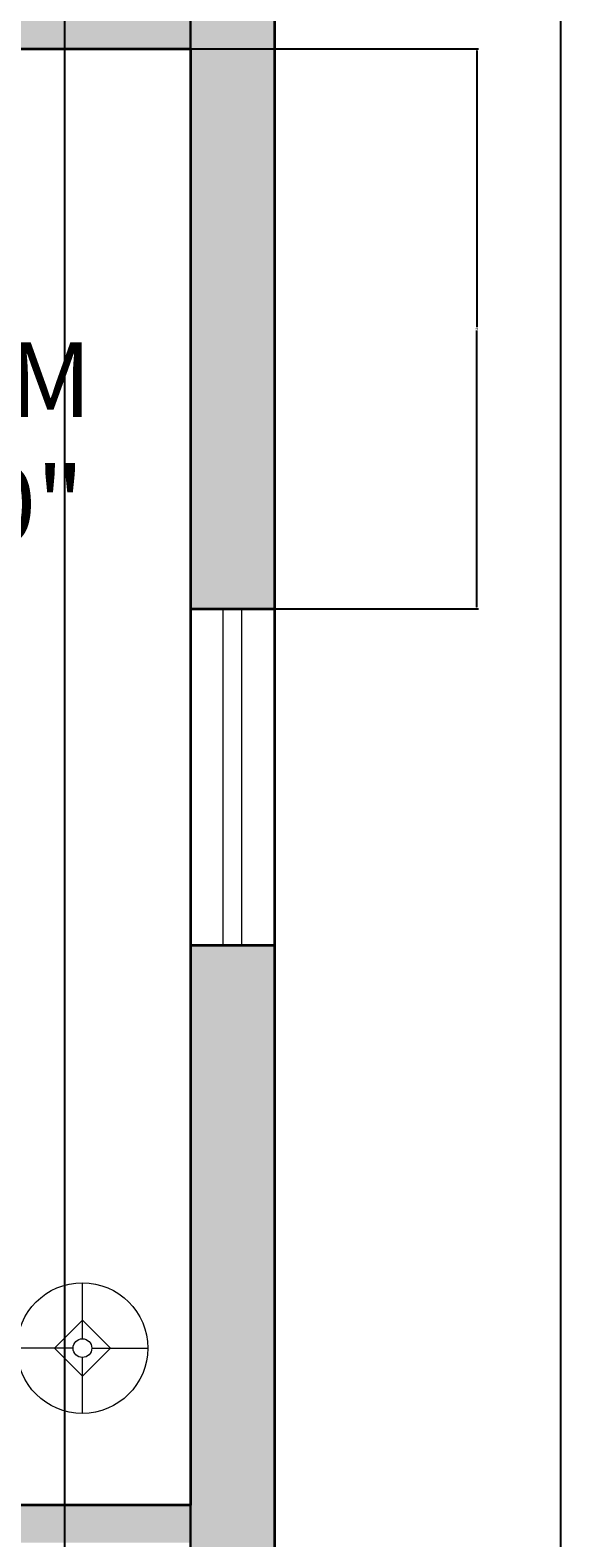
# Model space of a CAD drawing. Units: inches. Extents: x 1567 to 1964, y 1813 to 2447.
# Tile 6 of 28: x 1907 to 1964, y 1964 to 2125. Entities that reach past the tile are written whole.
import ezdxf

# ---------------------------------------------------------------- set-up
doc = ezdxf.new("R2010")
doc.units = ezdxf.units.IN
for name, color, linetype, lineweight in [('A-ANNO-DIMS', 2, 'Continuous', 18), ('A-AREA-IDEN', 7, 'Continuous', 18), ('A-FURN', 8, 'Continuous', 18), ('A-GLAZ', 4, 'Continuous', 18), ('A-WALL', 7, 'Continuous', 35)]:
    doc.layers.add(name, color=color, linetype=linetype, lineweight=lineweight)
doc.layers.add('A-FURN-PATT', color=252, linetype='Continuous', lineweight=13, true_color=0x939598)
doc.layers.add('A-WALL-PATT', color=251, linetype='Continuous', lineweight=13, true_color=0x636466)
doc.styles.get("Standard").update_dxf_attribs({"font": 'arial.ttf'})
doc.dimstyles.get("Standard").update_dxf_attribs({"dimtxt": 0.18, "dimasz": 0.18, "dimexe": 0.18, "dimexo": 0.0625, "dimgap": 0.09, "dimtad": 0, "dimtih": 1, "dimtoh": 1, "dimdec": 4, "dimzin": 0, "dimdsep": 46, "dimtxsty": 'Standard', "dimcen": 0.09, "dimadec": 0, "dimazin": 0, "dimtfac": 1, "dimtdec": 4, "dimtofl": 0, "dimtmove": 0, "dimatfit": 3, "dimfxl": 1, "dimtolj": 1, "dimtzin": 0, "dimarcsym": 0})

# ---------------------------------------------------------------- blocks, each defined once
blk = doc.blocks.new('Lamp - Table')
for p, q in [((0, 7), (0, 1)), ((0, 3), (-3, 0)), ((3, 0), (0, 3)), ((-1, 0), (-7, 0)), ((-3, 0), (0, -3)), ((0, -3), (3, 0)), ((1, 0), (7, 0)), ((0, -1), (0, -7))]:
    blk.add_line(p, q)
for radius in [7, 1]:
    blk.add_circle((0, 0), radius)
blk = doc.blocks.new('WINDOW-36IN')
for p, q in [((0, 2), (36, 2)), ((0, 0), (36, 0))]:
    blk.add_line(p, q)
blk = doc.blocks.new('*D40')
at = {"layer": 'A-ANNO-DIMS', "color": 0, "lineweight": -2, "transparency": 16777216}
for p, q in [((1933.49, 2416.29), (1964.26, 2416.29)), ((1964.08, 2416.11), (1964.08, 2130.47)), ((1964.08, 1844.47), (1964.08, 2130.11)), ((1933.49, 1844.29), (1964.26, 1844.29))]:
    blk.add_line(p, q, dxfattribs=at)
at = {"layer": 'A-ANNO-DIMS', "color": 0, "transparency": 16777216}
for points in [[(1964.05, 2416.11), (1964.11, 2416.11), (1964.08, 2416.29)], [(1964.05, 1844.47), (1964.11, 1844.47), (1964.08, 1844.29)]]:
    blk.add_solid(points, dxfattribs=at)
at = {"layer": 'Defpoints', "color": 0, "transparency": 16777216}
for p in [(1933.43, 2416.29), (1964.08, 2416.29), (1933.43, 1844.29)]:
    blk.add_point(p, dxfattribs=at)
at = {"layer": 'A-ANNO-DIMS', "color": 0, "transparency": 16777216, "insert": (1964.08, 2130.29), "char_height": 0.18, "attachment_point": 5}
blk.add_mtext('\\A1;572', dxfattribs=at)
blk = doc.blocks.new('*D52')
at = {"layer": 'A-ANNO-DIMS', "color": 0, "lineweight": -2, "transparency": 16777216}
for p, q in [((1924.49, 2123.29), (1955.26, 2123.29)), ((1955.08, 2123.11), (1955.08, 2093.47)), ((1955.08, 2063.47), (1955.08, 2093.11)), ((1924.49, 2063.29), (1955.26, 2063.29))]:
    blk.add_line(p, q, dxfattribs=at)
at = {"layer": 'A-ANNO-DIMS', "color": 0, "transparency": 16777216}
for points in [[(1955.05, 2123.11), (1955.11, 2123.11), (1955.08, 2123.29)], [(1955.05, 2063.47), (1955.11, 2063.47), (1955.08, 2063.29)]]:
    blk.add_solid(points, dxfattribs=at)
at = {"layer": 'Defpoints', "color": 0, "transparency": 16777216}
for p in [(1924.43, 2123.29), (1924.43, 2063.29), (1955.08, 2063.29)]:
    blk.add_point(p, dxfattribs=at)
at = {"layer": 'A-ANNO-DIMS', "color": 0, "transparency": 16777216, "insert": (1955.08, 2093.29), "char_height": 0.18, "attachment_point": 5}
blk.add_mtext('\\A1;60', dxfattribs=at)
blk = doc.blocks.new('*D71')
at = {"layer": 'A-ANNO-DIMS', "color": 0, "lineweight": -2, "transparency": 16777216}
for p, q in [((1799.43, 1910.75), (1799.43, 2447.12)), ((1799.61, 2446.94), (1861.65, 2446.94)), ((1924.25, 2446.94), (1862.21, 2446.94)), ((1924.43, 1910.75), (1924.43, 2447.12))]:
    blk.add_line(p, q, dxfattribs=at)
at = {"layer": 'A-ANNO-DIMS', "color": 0, "transparency": 16777216}
for points in [[(1799.61, 2446.97), (1799.61, 2446.91), (1799.43, 2446.94)], [(1924.25, 2446.97), (1924.25, 2446.91), (1924.43, 2446.94)]]:
    blk.add_solid(points, dxfattribs=at)
at = {"layer": 'Defpoints', "color": 0, "transparency": 16777216}
for p in [(1924.43, 2446.94), (1799.43, 1910.69), (1924.43, 1910.69)]:
    blk.add_point(p, dxfattribs=at)
at = {"layer": 'A-ANNO-DIMS', "color": 0, "transparency": 16777216, "insert": (1861.93, 2446.94), "char_height": 0.18, "attachment_point": 5}
blk.add_mtext('\\A1;125', dxfattribs=at)
blk = doc.blocks.new('*D72')
at = {"layer": 'A-ANNO-DIMS', "color": 0, "lineweight": -2, "transparency": 16777216}
for p, q in [((1910.93, 2175.23), (1910.93, 1813.46)), ((1924.43, 2175.23), (1924.43, 1813.46)), ((1911.11, 1813.64), (1917.36, 1813.64)), ((1924.25, 1813.64), (1918, 1813.64))]:
    blk.add_line(p, q, dxfattribs=at)
at = {"layer": 'A-ANNO-DIMS', "color": 0, "transparency": 16777216}
for points in [[(1911.11, 1813.67), (1911.11, 1813.61), (1910.93, 1813.64)], [(1924.25, 1813.67), (1924.25, 1813.61), (1924.43, 1813.64)]]:
    blk.add_solid(points, dxfattribs=at)
at = {"layer": 'Defpoints', "color": 0, "transparency": 16777216}
for p in [(1910.93, 2175.29), (1924.43, 2175.29), (1924.43, 1813.64)]:
    blk.add_point(p, dxfattribs=at)
at = {"layer": 'A-ANNO-DIMS', "color": 0, "transparency": 16777216, "insert": (1917.68, 1813.64), "char_height": 0.18, "attachment_point": 5}
blk.add_mtext('\\A1;13.5', dxfattribs=at)

msp = doc.modelspace()

# ---------------------------------------------------------------- hatches: boundary and pattern name
at = {"layer": 'A-FURN-PATT'}
h = msp.add_hatch(color=256, dxfattribs=at)
h.dxf.hatch_style = 1
h.paths.add_polyline_path([(1697.3402, 2374.8316), (1682.1402, 2374.8316), (1682.1402, 2387.6316), (1637.3402, 2387.6316), (1637.3402, 2324.4315), (1697.3402, 2324.4315)])
h.paths.add_polyline_path([(1891.1093, 2375.8204), (1875.9094, 2375.8204), (1875.9094, 2388.6204), (1831.1094, 2388.6204), (1831.1094, 2325.4204), (1891.1093, 2325.4204)])
h.paths.add_polyline_path([(1702.5611, 2206.8057), (1702.5611, 2210.8057), (1699.7395, 2209.9436), (1697.013, 2209.2403), (1694.3857, 2208.6763), (1691.8615, 2208.2326), (1689.4443, 2207.8896), (1687.1381, 2207.6282), (1684.9469, 2207.4289), (1682.8747, 2207.2725), (1680.9233, 2207.1425), (1679.0865, 2207.0339), (1677.3558, 2206.9445), (1675.7229, 2206.8719), (1674.1794, 2206.8141), (1672.7169, 2206.7688), (1671.327, 2206.7339), (1670.0014, 2206.707), (1668.7314, 2206.6866), (1667.5072, 2206.6732), (1666.3188, 2206.668), (1665.1561, 2206.6722), (1664.009, 2206.6869), (1662.8675, 2206.7133), (1661.7215, 2206.7525), (1660.5611, 2206.8057), (1660.5611, 2202.8057), (1661.9932, 2202.9556), (1663.3314, 2203.0744), (1664.5899, 2203.1671), (1665.7831, 2203.2385), (1666.9254, 2203.2935), (1668.0311, 2203.3368), (1669.1145, 2203.3734), (1670.1902, 2203.4081), (1671.2724, 2203.4451), (1672.3759, 2203.4866), (1673.5155, 2203.534), (1674.706, 2203.5887), (1675.9621, 2203.6523), (1677.2986, 2203.7262), (1678.7304, 2203.8118), (1680.2722, 2203.9108), (1681.947, 2204.0272), (1683.8108, 2204.1769), (1685.9279, 2204.3782), (1688.3626, 2204.6496), (1691.179, 2205.0096), (1694.4413, 2205.4767), (1698.214, 2206.0692)])
h.paths.add_polyline_path([(1702.5611, 2218.8057), (1701.9821, 2217.9383), (1701.3316, 2217.191), (1700.6091, 2216.5515), (1699.8141, 2216.0071), (1698.946, 2215.5454), (1698.0041, 2215.1536), (1696.9879, 2214.8194), (1695.8969, 2214.5301), (1694.7328, 2214.2753), (1693.5072, 2214.0522), (1692.2339, 2213.8602), (1690.9266, 2213.6989), (1689.5994, 2213.5675), (1688.266, 2213.4654), (1686.9402, 2213.392), (1685.636, 2213.3467), (1684.3619, 2213.3287), (1683.1053, 2213.3361), (1681.8482, 2213.3668), (1680.5727, 2213.4187), (1679.2608, 2213.4898), (1677.8948, 2213.5779), (1676.4565, 2213.6811), (1674.9282, 2213.7971), (1673.2982, 2213.9236), (1671.5804, 2214.0573), (1669.795, 2214.1945), (1667.9622, 2214.3316), (1666.1022, 2214.4649), (1664.2352, 2214.5908), (1662.3814, 2214.7056), (1660.5611, 2214.8057), (1660.5611, 2206.8057), (1661.7215, 2206.7525), (1662.8675, 2206.7133), (1664.009, 2206.6869), (1665.1561, 2206.6722), (1666.3188, 2206.668), (1667.5072, 2206.6732), (1668.7314, 2206.6866), (1670.0014, 2206.707), (1671.327, 2206.7339), (1672.7169, 2206.7688), (1674.1794, 2206.8141), (1675.7229, 2206.8719), (1677.3558, 2206.9445), (1679.0865, 2207.0339), (1680.9233, 2207.1425), (1682.8747, 2207.2725), (1684.9469, 2207.4289), (1687.1381, 2207.6282), (1689.4443, 2207.8896), (1691.8615, 2208.2326), (1694.3857, 2208.6763), (1697.013, 2209.2403), (1699.7395, 2209.9436), (1702.5611, 2210.8057)])
h.paths.add_polyline_path([(1700.6091, 2216.5515), (1701.3316, 2217.191), (1701.9821, 2217.9383), (1702.5611, 2218.8057), (1702.5611, 2222.8057), (1689.452, 2222.8057), (1689.0171, 2222.4556), (1688.4521, 2222.0354), (1687.7806, 2221.5662), (1687.0235, 2221.067), (1686.2019, 2220.5566), (1685.3367, 2220.0541), (1684.4491, 2219.5785), (1683.56, 2219.1486), (1682.6867, 2218.7795), (1681.8312, 2218.4692), (1680.9918, 2218.212), (1680.1667, 2218.0019), (1679.3541, 2217.833), (1678.5524, 2217.6995), (1677.7597, 2217.5954), (1676.9744, 2217.5149), (1676.1942, 2217.4531), (1675.4146, 2217.4093), (1674.6309, 2217.384), (1673.8381, 2217.3774), (1673.0313, 2217.39), (1672.2056, 2217.4221), (1671.3562, 2217.4741), (1670.4782, 2217.5463), (1669.5642, 2217.639), (1668.5968, 2217.7516), (1667.5562, 2217.8833), (1666.4226, 2218.0336), (1665.1761, 2218.2017), (1663.7969, 2218.3869), (1662.2651, 2218.5885), (1660.5611, 2218.8057), (1660.5611, 2214.8057), (1662.3814, 2214.7056), (1664.2352, 2214.5908), (1666.1022, 2214.4649), (1667.9622, 2214.3316), (1669.795, 2214.1945), (1671.5804, 2214.0573), (1673.2982, 2213.9236), (1674.9282, 2213.7971), (1676.4565, 2213.6811), (1677.8948, 2213.5779), (1679.2608, 2213.4898), (1680.5727, 2213.4187), (1681.8482, 2213.3668), (1683.1053, 2213.3361), (1684.3619, 2213.3287), (1685.636, 2213.3467), (1686.9402, 2213.392), (1688.266, 2213.4654), (1689.5994, 2213.5675), (1690.9266, 2213.6989), (1692.2339, 2213.8602), (1693.5072, 2214.0522), (1694.7328, 2214.2753), (1695.8969, 2214.5301), (1696.9879, 2214.8194), (1698.0041, 2215.1536), (1698.946, 2215.5454), (1699.8141, 2216.0071)])
h.paths.add_polyline_path([(1687.0235, 2221.067), (1687.7806, 2221.5662), (1688.4521, 2222.0354), (1689.0171, 2222.4556), (1689.452, 2222.8057), (1660.5611, 2222.8057), (1660.5611, 2218.8057), (1662.2651, 2218.5885), (1663.7969, 2218.3869), (1665.1761, 2218.2017), (1666.4226, 2218.0336), (1667.5562, 2217.8833), (1668.5968, 2217.7516), (1669.5642, 2217.639), (1670.4782, 2217.5463), (1671.3562, 2217.4741), (1672.2056, 2217.4221), (1673.0313, 2217.39), (1673.8381, 2217.3774), (1674.6309, 2217.384), (1675.4146, 2217.4093), (1676.1942, 2217.4531), (1676.9744, 2217.5149), (1677.7597, 2217.5954), (1678.5524, 2217.6995), (1679.3541, 2217.833), (1680.1667, 2218.0019), (1680.9918, 2218.212), (1681.8312, 2218.4692), (1682.6867, 2218.7795), (1683.56, 2219.1486), (1684.4491, 2219.5785), (1685.3367, 2220.0541), (1686.2019, 2220.5566)], flags=17)
h.paths.add_polyline_path([(1702.5611, 2198.8057), (1698.9289, 2199.2412), (1695.8472, 2199.5774), (1693.2166, 2199.8257), (1690.9377, 2199.9973), (1688.9111, 2200.1033), (1687.0375, 2200.155), (1685.2174, 2200.1637), (1683.3514, 2200.1406), (1681.3514, 2200.0941), (1679.1736, 2200.0225), (1676.7858, 2199.921), (1674.1554, 2199.7852), (1671.2502, 2199.6103), (1668.0377, 2199.3919), (1664.4854, 2199.1252), (1660.5611, 2198.8057), (1660.5611, 2194.8057), (1662.2697, 2194.9771), (1663.9673, 2195.0999), (1665.6339, 2195.1809), (1667.2495, 2195.227), (1668.7941, 2195.2449), (1670.2478, 2195.2414), (1671.5906, 2195.2233), (1672.8026, 2195.1974), (1673.8739, 2195.1689), (1674.8359, 2195.1364), (1675.7302, 2195.0967), (1676.5982, 2195.0469), (1677.4817, 2194.9838), (1678.422, 2194.9043), (1679.4609, 2194.8055), (1680.6397, 2194.6842), (1682.005, 2194.5341), (1683.6223, 2194.335), (1685.562, 2194.0637), (1687.8945, 2193.6967), (1690.6902, 2193.2108), (1694.0196, 2192.5826), (1697.9531, 2191.7887), (1702.5611, 2190.8057)])
h.paths.add_polyline_path([(1702.5611, 2206.8057), (1698.214, 2206.0692), (1694.4413, 2205.4767), (1691.179, 2205.0096), (1688.3626, 2204.6496), (1685.9279, 2204.3782), (1683.8108, 2204.1769), (1681.947, 2204.0272), (1680.2722, 2203.9108), (1678.7304, 2203.8118), (1677.2986, 2203.7262), (1675.9621, 2203.6523), (1674.706, 2203.5887), (1673.5155, 2203.534), (1672.3759, 2203.4866), (1671.2724, 2203.4451), (1670.1902, 2203.4081), (1669.1145, 2203.3734), (1668.0311, 2203.3368), (1666.9254, 2203.2935), (1665.7831, 2203.2385), (1664.5899, 2203.1671), (1663.3314, 2203.0744), (1661.9932, 2202.9556), (1660.5611, 2202.8057), (1660.5611, 2198.8057), (1664.4854, 2199.1252), (1668.0377, 2199.3919), (1671.2502, 2199.6103), (1674.1554, 2199.7852), (1676.7858, 2199.921), (1679.1736, 2200.0225), (1681.3514, 2200.0941), (1683.3514, 2200.1406), (1685.2174, 2200.1637), (1687.0375, 2200.155), (1688.9111, 2200.1033), (1690.9377, 2199.9973), (1693.2166, 2199.8257), (1695.8472, 2199.5774), (1698.9289, 2199.2412), (1702.5611, 2198.8057)])
h.paths.add_polyline_path([(1702.5611, 2190.8057), (1697.9531, 2191.7887), (1694.0196, 2192.5826), (1690.6902, 2193.2108), (1687.8945, 2193.6967), (1685.562, 2194.0637), (1683.6223, 2194.335), (1682.005, 2194.5341), (1680.6397, 2194.6842), (1679.4609, 2194.8055), (1678.422, 2194.9043), (1677.4817, 2194.9838), (1676.5982, 2195.0469), (1675.7302, 2195.0967), (1674.8359, 2195.1364), (1673.8739, 2195.1689), (1672.8026, 2195.1974), (1671.5906, 2195.2233), (1670.2478, 2195.2414), (1668.7941, 2195.2449), (1667.2495, 2195.227), (1665.6339, 2195.1809), (1663.9673, 2195.0999), (1662.2697, 2194.9771), (1660.5611, 2194.8057), (1660.5611, 2190.8057), (1665.9637, 2190.2699), (1670.5105, 2189.7867), (1674.3035, 2189.3504), (1677.4445, 2188.9552), (1680.0354, 2188.5951), (1682.1782, 2188.2644), (1683.9747, 2187.9571), (1685.5268, 2187.6675), (1686.9225, 2187.3901), (1688.1943, 2187.1216), (1689.3606, 2186.859), (1690.4399, 2186.5993), (1691.4508, 2186.3396), (1692.4118, 2186.0769), (1693.3413, 2185.8084), (1694.2579, 2185.531), (1695.1786, 2185.2422), (1696.1142, 2184.9406), (1697.0739, 2184.6252), (1698.0671, 2184.2949), (1699.1032, 2183.9489), (1700.1913, 2183.586), (1701.3408, 2183.2053), (1702.5611, 2182.8057)])
h.paths.add_polyline_path([(1702.5611, 2182.8057), (1701.3408, 2183.2053), (1700.1913, 2183.586), (1699.1032, 2183.9489), (1698.0671, 2184.2949), (1697.0739, 2184.6252), (1696.1142, 2184.9406), (1695.1786, 2185.2422), (1694.2579, 2185.531), (1693.3413, 2185.8084), (1692.4118, 2186.0769), (1691.4508, 2186.3396), (1690.4399, 2186.5993), (1689.3606, 2186.859), (1688.1943, 2187.1216), (1686.9225, 2187.3901), (1685.5268, 2187.6675), (1683.9747, 2187.9571), (1682.1782, 2188.2644), (1680.0354, 2188.5951), (1677.4445, 2188.9552), (1674.3035, 2189.3504), (1670.5105, 2189.7867), (1665.9637, 2190.2699), (1660.5611, 2190.8057), (1660.5611, 2186.8057), (1663.5709, 2186.52), (1666.0965, 2186.2414), (1668.1979, 2185.9698), (1669.9351, 2185.7048), (1671.3681, 2185.446), (1672.5568, 2185.1931), (1673.5613, 2184.9458), (1674.4415, 2184.7037), (1675.2485, 2184.4664), (1675.9976, 2184.2328), (1677.0295, 2183.8907), (1678.2492, 2183.4332), (1679.354, 2182.9669), (1680.4123, 2182.4724), (1681.3757, 2181.9718), (1682.2435, 2181.4594), (1683.1864, 2180.8057), (1702.5611, 2180.8057)])
h.paths.add_polyline_path([(1677.3469, 2183.7716), (1676.6949, 2184.0016), (1675.9976, 2184.2328), (1675.2485, 2184.4664), (1674.4415, 2184.7037), (1673.5613, 2184.9458), (1672.5568, 2185.1931), (1671.3681, 2185.446), (1669.9351, 2185.7048), (1668.1979, 2185.9698), (1666.0965, 2186.2414), (1663.5709, 2186.52), (1660.5611, 2186.8057), (1660.5611, 2180.8057), (1683.1506, 2180.8057), (1682.802, 2181.0722), (1682.4264, 2181.3326), (1682.0201, 2181.5913), (1681.586, 2181.8476), (1681.1268, 2182.1011), (1680.6453, 2182.3513), (1680.1443, 2182.5976), (1679.6266, 2182.8395), (1679.0933, 2183.0769), (1678.5398, 2183.3105), (1677.9598, 2183.5417)], flags=17)
h.paths.add_polyline_path([(1824.4511, 2199.9016), (1824.089, 2199.9302), (1824.0595, 2199.9372), (1824.0397, 2199.9406), (1823.5413, 2200.0576), (1823.4095, 2200.0864), (1823.0664, 2200.1559), (1822.6419, 2200.2361), (1822.1519, 2200.3222), (1821.6126, 2200.4093), (1821.0401, 2200.4925), (1820.4505, 2200.5669), (1819.8599, 2200.6276), (1819.2845, 2200.6697), (1818.7366, 2200.6896), (1818.2141, 2200.688), (1817.7112, 2200.6668), (1817.222, 2200.6281), (1816.7405, 2200.5737), (1816.261, 2200.5057), (1815.7776, 2200.4259), (1815.2845, 2200.3364), (1814.3007, 2200.149), (1813.3315, 2199.9765), (1812.406, 2199.8514), (1811.6868, 2199.7739), (1810.8992, 2199.7121), (1810.0345, 2199.6697), (1809.0854, 2199.6497), (1808.0514, 2199.6502), (1806.9334, 2199.6683), (1805.7324, 2199.701), (1804.4493, 2199.7454), (1803.0852, 2199.7986), (1801.641, 2199.8577), (1800.1178, 2199.9197), (1798.5134, 2199.9818), (1796.8144, 2200.0415), (1795.004, 2200.0962), (1793.0657, 2200.1437), (1790.9828, 2200.1814), (1788.7389, 2200.2068), (1786.3171, 2200.2177), (1783.7011, 2200.2114), (1780.8715, 2200.185), (1777.7988, 2200.1326), (1774.4506, 2200.0481), (1770.7948, 2199.9249), (1766.7992, 2199.7569), (1762.4316, 2199.5376), (1757.6596, 2199.2606), (1752.4511, 2198.9197), (1752.4511, 2193.4197), (1761.2668, 2193.6071), (1768.3671, 2193.7934), (1773.9821, 2193.9778), (1778.3417, 2194.1593), (1781.6759, 2194.3369), (1784.2148, 2194.5096), (1786.1882, 2194.6764), (1787.8261, 2194.8364), (1789.3219, 2194.9887), (1790.7226, 2195.1333), (1792.0383, 2195.27), (1793.2792, 2195.3989), (1794.4557, 2195.52), (1795.5781, 2195.6333), (1796.6564, 2195.7387), (1797.7011, 2195.8364), (1798.7216, 2195.9259), (1799.7245, 2196.0057), (1800.7158, 2196.0737), (1801.7011, 2196.1281), (1802.6865, 2196.1668), (1803.6777, 2196.188), (1804.6806, 2196.1896), (1805.7011, 2196.1697), (1806.7423, 2196.1273), (1807.7962, 2196.0643), (1808.852, 2195.9837), (1809.899, 2195.8885), (1810.9265, 2195.7815), (1811.9238, 2195.6658), (1812.88, 2195.5442), (1813.7845, 2195.4197), (1814.6296, 2195.2948), (1815.4205, 2195.1704), (1816.1656, 2195.0469), (1816.873, 2194.9249), (1817.5511, 2194.8049), (1818.2083, 2194.6873), (1818.8527, 2194.5726), (1819.4928, 2194.4614), (1820.1348, 2194.3554), (1820.7773, 2194.2615), (1821.4169, 2194.1882), (1822.0501, 2194.1437), (1822.6735, 2194.1363), (1823.2838, 2194.1743), (1823.8775, 2194.266), (1824.4511, 2194.4197)])
h.paths.add_polyline_path([(1821.4716, 2190.5098), (1820.4303, 2190.5708), (1819.3811, 2190.6415), (1818.3339, 2190.7186), (1817.2985, 2190.7986), (1816.2845, 2190.8781), (1815.2976, 2190.9542), (1814.3274, 2191.0259), (1813.3592, 2191.0927), (1812.3782, 2191.1541), (1811.3699, 2191.2097), (1810.3196, 2191.2589), (1809.2127, 2191.3013), (1808.0345, 2191.3364), (1806.7708, 2191.3634), (1805.4094, 2191.3807), (1803.9387, 2191.3862), (1802.3469, 2191.3781), (1800.6223, 2191.3543), (1798.7532, 2191.313), (1796.7278, 2191.2521), (1794.5344, 2191.1697), (1792.128, 2191.0648), (1789.33, 2190.9393), (1785.9285, 2190.7962), (1781.7115, 2190.6385), (1776.4672, 2190.469), (1769.9836, 2190.2908), (1762.0489, 2190.1067), (1752.4511, 2189.9197), (1752.4511, 2185.4197), (1758.363, 2185.5846), (1763.4179, 2185.7075), (1767.7199, 2185.7933), (1771.373, 2185.8468), (1774.4811, 2185.873), (1777.1484, 2185.8768), (1779.4787, 2185.8629), (1781.5761, 2185.8364), (1783.5287, 2185.8014), (1785.3606, 2185.7596), (1787.0802, 2185.7119), (1788.6959, 2185.6593), (1790.2158, 2185.6028), (1791.6484, 2185.5434), (1793.0018, 2185.4821), (1794.2844, 2185.4197), (1795.5065, 2185.3576), (1796.6861, 2185.298), (1797.8433, 2185.2432), (1798.998, 2185.1958), (1800.1703, 2185.1581), (1801.3801, 2185.1326), (1802.6476, 2185.1218), (1803.9928, 2185.1281), (1805.4444, 2185.1555), (1807.0663, 2185.2147), (1808.9315, 2185.3178), (1811.1126, 2185.477), (1813.6823, 2185.7046), (1816.7135, 2186.0128), (1820.2788, 2186.4138), (1824.4511, 2186.9197), (1824.4511, 2190.4197), (1823.4918, 2190.4309), (1822.4954, 2190.4621)])
h.paths.add_polyline_path([(1797.3762, 2216.0584), (1797.6199, 2216.2267), (1797.9558, 2216.3355), (1798.3017, 2216.3703), (1798.5761, 2216.3781), (1798.8974, 2216.3703), (1799.2714, 2216.3468), (1799.704, 2216.3078), (1800.2011, 2216.2531), (1800.7695, 2216.1829), (1801.4205, 2216.0981), (1802.1662, 2215.9996), (1803.0188, 2215.8885), (1803.9906, 2215.7656), (1805.0937, 2215.632), (1806.3404, 2215.4886), (1807.7428, 2215.3364), (1809.3101, 2215.1764), (1811.039, 2215.0096), (1812.9232, 2214.8369), (1814.9563, 2214.6593), (1817.132, 2214.4778), (1819.444, 2214.2934), (1821.8858, 2214.1071), (1824.4511, 2213.9197), (1824.4511, 2217.9197), (1752.4511, 2217.9197), (1752.4511, 2214.9197), (1757.2739, 2214.8973), (1761.6432, 2214.8338), (1765.5973, 2214.7352), (1769.1751, 2214.6072), (1772.4149, 2214.4559), (1775.3554, 2214.2869), (1778.0352, 2214.1063), (1780.4928, 2213.9197), (1782.7607, 2213.7329), (1784.8476, 2213.5499), (1786.7557, 2213.3748), (1788.4876, 2213.2114), (1790.0456, 2213.0636), (1791.4322, 2212.9354), (1792.6499, 2212.8305), (1793.7011, 2212.7531), (1794.5904, 2212.7059), (1795.3313, 2212.688), (1795.9394, 2212.6974), (1796.4303, 2212.7322), (1796.8196, 2212.7905), (1797.123, 2212.8703), (1797.356, 2212.9695), (1797.5344, 2213.0864), (1797.6716, 2213.2187), (1797.7727, 2213.3637), (1797.8406, 2213.5185), (1797.8782, 2213.6801), (1797.8884, 2213.8457), (1797.8743, 2214.0122), (1797.8386, 2214.1767), (1797.7844, 2214.3364), (1797.7149, 2214.4889), (1797.6347, 2214.6346), (1797.5486, 2214.7744), (1797.3327, 2215.109), (1797.178, 2215.4303), (1797.1896, 2215.7939)])
h.paths.add_polyline_path([(1804.7872, 2210.6789), (1804.546, 2211.022), (1804.3512, 2211.3917), (1804.2466, 2211.7546), (1804.2574, 2212.0998), (1804.4058, 2212.4178), (1804.7068, 2212.7007), (1805.1359, 2212.9124), (1805.5279, 2212.9926), (1805.8136, 2213.0154), (1806.1178, 2213.0031), (1806.4405, 2212.9529), (1806.7929, 2212.867), (1807.1893, 2212.7489), (1807.6438, 2212.602), (1808.1706, 2212.4297), (1808.7838, 2212.2355), (1809.4976, 2212.0227), (1810.3261, 2211.7947), (1811.2868, 2211.5533), (1812.4101, 2211.2928), (1813.7297, 2211.0059), (1815.2793, 2210.6854), (1817.0925, 2210.3238), (1819.2031, 2209.9139), (1821.6447, 2209.4483), (1824.4511, 2208.9197), (1824.4511, 2213.9197), (1821.8858, 2214.1071), (1819.444, 2214.2934), (1817.132, 2214.4778), (1814.9563, 2214.6593), (1812.9232, 2214.8369), (1811.039, 2215.0096), (1809.3101, 2215.1764), (1807.7428, 2215.3364), (1806.3404, 2215.4886), (1805.0937, 2215.632), (1803.9906, 2215.7656), (1803.0188, 2215.8885), (1802.1662, 2215.9996), (1801.4205, 2216.0981), (1800.7695, 2216.1829), (1800.2011, 2216.2531), (1799.704, 2216.3078), (1799.2714, 2216.3468), (1798.8974, 2216.3703), (1798.5761, 2216.3781), (1798.3017, 2216.3703), (1798.0683, 2216.3468), (1797.87, 2216.3078), (1797.7011, 2216.2531), (1797.5566, 2216.1831), (1797.4355, 2216.0994), (1797.3378, 2216.004), (1797.2636, 2215.8989), (1797.2128, 2215.7859), (1797.1855, 2215.6671), (1797.1816, 2215.5444), (1797.2011, 2215.4197), (1797.2433, 2215.2946), (1797.304, 2215.1684), (1797.3783, 2215.0403), (1797.4615, 2214.9093), (1797.6718, 2214.5836), (1797.8218, 2214.2545), (1797.8933, 2213.9247), (1797.8728, 2213.5918), (1797.7366, 2213.2814), (1797.4586, 2213.0132), (1797.123, 2212.8703), (1796.8196, 2212.7905), (1796.4303, 2212.7322), (1795.9394, 2212.6974), (1795.3313, 2212.688), (1794.5904, 2212.7059), (1793.7011, 2212.7531), (1792.6499, 2212.8305), (1791.4322, 2212.9354), (1790.0456, 2213.0636), (1788.4876, 2213.2114), (1786.7557, 2213.3748), (1784.8476, 2213.5499), (1782.7607, 2213.7329), (1780.4928, 2213.9197), (1778.0352, 2214.1063), (1775.3554, 2214.2869), (1772.4149, 2214.4559), (1769.1751, 2214.6072), (1765.5973, 2214.7352), (1761.6432, 2214.8338), (1757.2739, 2214.8973), (1752.4511, 2214.9197), (1752.4511, 2209.9197), (1759.4745, 2210.0625), (1765.2786, 2210.1242), (1770.027, 2210.1175), (1773.8834, 2210.0551), (1777.0112, 2209.9498), (1779.5741, 2209.8143), (1781.7357, 2209.6611), (1783.6594, 2209.5031), (1785.4813, 2209.3506), (1787.2265, 2209.2049), (1788.8926, 2209.0651), (1790.4771, 2208.9301), (1791.9777, 2208.7991), (1793.3919, 2208.671), (1794.7171, 2208.5449), (1795.9511, 2208.4197), (1797.0922, 2208.2952), (1798.1425, 2208.1736), (1799.1049, 2208.0579), (1799.9823, 2207.951), (1800.7778, 2207.8558), (1801.4941, 2207.7752), (1802.1342, 2207.7122), (1802.7011, 2207.6697), (1803.1982, 2207.65), (1803.6308, 2207.6528), (1804.0048, 2207.6771), (1804.3261, 2207.7218), (1804.6005, 2207.7861), (1804.8339, 2207.869), (1805.0322, 2207.9694), (1805.2011, 2208.0864), (1805.3455, 2208.2189), (1805.4654, 2208.365), (1805.56, 2208.5229), (1805.6282, 2208.6906), (1805.6691, 2208.866), (1805.6816, 2209.0473), (1805.6648, 2209.2326), (1805.6178, 2209.4197), (1805.5406, 2209.6072), (1805.4381, 2209.7947), (1805.316, 2209.9822), (1805.1803, 2210.1697), (1805.0367, 2210.3572)])
h.paths.add_polyline_path([(1801.4941, 2207.7752), (1800.7778, 2207.8558), (1799.9823, 2207.951), (1799.1049, 2208.0579), (1798.1425, 2208.1736), (1797.0922, 2208.2952), (1795.9511, 2208.4197), (1794.7171, 2208.5449), (1793.3919, 2208.671), (1791.9777, 2208.7991), (1790.4771, 2208.9301), (1788.8926, 2209.0651), (1787.2265, 2209.2049), (1785.4813, 2209.3506), (1783.6594, 2209.5031), (1781.7357, 2209.6611), (1779.5741, 2209.8143), (1777.0112, 2209.9498), (1773.8834, 2210.0551), (1770.027, 2210.1175), (1765.2786, 2210.1242), (1759.4745, 2210.0625), (1752.4511, 2209.9197), (1752.4511, 2205.4197), (1757.7354, 2205.2545), (1762.3821, 2205.1294), (1766.4565, 2205.0374), (1770.024, 2204.9718), (1773.1502, 2204.9258), (1775.9003, 2204.8924), (1778.3399, 2204.8649), (1780.5344, 2204.8364), (1782.5421, 2204.8014), (1784.3925, 2204.7596), (1786.1082, 2204.7119), (1787.7115, 2204.6593), (1789.225, 2204.6028), (1790.6711, 2204.5434), (1792.0724, 2204.4821), (1793.4511, 2204.4197), (1794.8241, 2204.3576), (1796.1855, 2204.2973), (1797.5234, 2204.241), (1798.8261, 2204.1906), (1800.082, 2204.1479), (1801.2792, 2204.115), (1802.4062, 2204.0939), (1803.4511, 2204.0864), (1804.4051, 2204.0942), (1805.2701, 2204.1176), (1806.0512, 2204.1567), (1806.7532, 2204.2114), (1807.381, 2204.2817), (1807.9394, 2204.3676), (1808.4334, 2204.4692), (1808.8678, 2204.5864), (1809.248, 2204.7187), (1809.5813, 2204.8637), (1809.8756, 2205.0185), (1810.1386, 2205.1801), (1810.3782, 2205.3457), (1810.6022, 2205.5122), (1810.9725, 2205.7941), (1811.3803, 2206.072), (1811.739, 2206.2612), (1812.0032, 2206.3781), (1812.2869, 2206.4793), (1812.5931, 2206.563), (1812.9246, 2206.6271), (1813.2845, 2206.6697), (1813.6746, 2206.6894), (1814.0931, 2206.6867), (1814.5369, 2206.6624), (1815.0032, 2206.6176), (1815.489, 2206.5534), (1815.9915, 2206.4705), (1816.5076, 2206.3701), (1817.0345, 2206.2531), (1817.5753, 2206.1196), (1818.1582, 2205.9666), (1818.8172, 2205.7902), (1819.5865, 2205.5864), (1820.5004, 2205.3514), (1821.5931, 2205.0812), (1822.8986, 2204.7719), (1824.4511, 2204.4197), (1824.4511, 2208.9197), (1821.6447, 2209.4483), (1819.2031, 2209.9139), (1817.0925, 2210.3238), (1815.2793, 2210.6854), (1813.7297, 2211.0059), (1812.4101, 2211.2928), (1811.2868, 2211.5533), (1810.3261, 2211.7947), (1809.4976, 2212.0227), (1808.7838, 2212.2355), (1808.1706, 2212.4297), (1807.6438, 2212.602), (1807.1893, 2212.7489), (1806.7929, 2212.867), (1806.4405, 2212.9529), (1806.1178, 2213.0031), (1805.8136, 2213.0154), (1805.5279, 2212.9926), (1805.2638, 2212.9386), (1805.024, 2212.8572), (1804.8116, 2212.7524), (1804.6295, 2212.6281), (1804.4806, 2212.4881), (1804.3678, 2212.3364), (1804.2931, 2212.1764), (1804.2545, 2212.0096), (1804.2491, 2211.8369), (1804.274, 2211.6593), (1804.3263, 2211.4778), (1804.4029, 2211.2934), (1804.5011, 2211.1071), (1804.6178, 2210.9197), (1804.7496, 2210.7322), (1804.8912, 2210.5447), (1805.154, 2210.2061), (1805.3962, 2209.8715), (1805.5964, 2209.5053), (1805.688, 2209.1402), (1805.6629, 2208.7758), (1805.5257, 2208.4385), (1805.2839, 2208.1437), (1804.9434, 2207.9078), (1804.6005, 2207.7861), (1804.3261, 2207.7218), (1804.0048, 2207.6771), (1803.6308, 2207.6528), (1803.1982, 2207.65), (1802.7011, 2207.6697), (1802.1342, 2207.7122)])
h.paths.add_polyline_path([(1824.4511, 2204.4197), (1822.8986, 2204.7719), (1821.5931, 2205.0812), (1820.5004, 2205.3514), (1819.5865, 2205.5864), (1818.8172, 2205.7902), (1818.1582, 2205.9666), (1817.5753, 2206.1196), (1817.0345, 2206.2531), (1816.5076, 2206.3701), (1815.9915, 2206.4705), (1815.489, 2206.5534), (1815.0032, 2206.6176), (1814.5369, 2206.6624), (1814.0931, 2206.6867), (1813.6746, 2206.6894), (1813.2845, 2206.6697), (1812.9246, 2206.6271), (1812.5931, 2206.563), (1812.2869, 2206.4793), (1812.0032, 2206.3781), (1811.739, 2206.2612), (1811.4915, 2206.1307), (1811.2576, 2205.9884), (1811.0345, 2205.8364), (1810.8183, 2205.6767), (1810.4357, 2205.3854), (1810.1386, 2205.1801), (1809.8756, 2205.0185), (1809.5813, 2204.8637), (1809.248, 2204.7187), (1808.8678, 2204.5864), (1808.4334, 2204.4692), (1807.9394, 2204.3676), (1807.381, 2204.2817), (1806.7532, 2204.2114), (1806.0512, 2204.1567), (1805.2701, 2204.1176), (1804.4051, 2204.0942), (1803.4511, 2204.0864), (1802.4062, 2204.0939), (1801.2792, 2204.115), (1800.082, 2204.1479), (1798.8261, 2204.1906), (1797.5234, 2204.241), (1796.1855, 2204.2973), (1794.8241, 2204.3576), (1793.4511, 2204.4197), (1792.0724, 2204.4821), (1790.6711, 2204.5434), (1789.225, 2204.6028), (1787.7115, 2204.6593), (1786.1082, 2204.7119), (1784.3925, 2204.7596), (1782.5421, 2204.8014), (1780.5344, 2204.8364), (1778.3399, 2204.8649), (1775.9003, 2204.8924), (1773.1502, 2204.9258), (1770.024, 2204.9718), (1766.4565, 2205.0374), (1762.3821, 2205.1294), (1757.7354, 2205.2545), (1752.4511, 2205.4197), (1752.4511, 2198.9197), (1757.6596, 2199.2606), (1762.4316, 2199.5376), (1766.7992, 2199.7569), (1770.7948, 2199.9249), (1774.4506, 2200.0481), (1777.7988, 2200.1326), (1780.8715, 2200.185), (1783.7011, 2200.2114), (1786.3171, 2200.2177), (1788.7389, 2200.2068), (1790.9828, 2200.1814), (1793.0657, 2200.1437), (1795.004, 2200.0962), (1796.8144, 2200.0415), (1798.5134, 2199.9818), (1800.1178, 2199.9197), (1801.641, 2199.8577), (1803.0852, 2199.7986), (1804.4493, 2199.7454), (1805.7324, 2199.701), (1806.9334, 2199.6683), (1808.0514, 2199.6502), (1809.0854, 2199.6497), (1810.0345, 2199.6697), (1810.8992, 2199.7121), (1811.6868, 2199.7739), (1812.406, 2199.8514), (1813.0657, 2199.9406), (1813.6746, 2200.0376), (1814.2415, 2200.1385), (1814.7752, 2200.2394), (1815.2845, 2200.3364), (1815.7776, 2200.4259), (1816.261, 2200.5057), (1816.7405, 2200.5737), (1817.222, 2200.6281), (1817.7112, 2200.6668), (1818.2141, 2200.688), (1818.7366, 2200.6896), (1819.2845, 2200.6697), (1819.8599, 2200.6276), (1820.4505, 2200.5669), (1821.0401, 2200.4925), (1821.6126, 2200.4093), (1822.1519, 2200.3222), (1822.6419, 2200.2361), (1823.0664, 2200.1559), (1823.5408, 2200.0598), (1824.0595, 2199.9372), (1824.1105, 2199.9285), (1824.1888, 2199.9223), (1824.2953, 2199.9201), (1824.4511, 2199.9197)])
h.paths.add_polyline_path([(1795.4295, 2021.5492), (1771.4295, 2021.5492), (1771.4295, 1988.29), (1735.4295, 1988.29), (1735.4295, 2055.79), (1711.4295, 2055.79), (1711.4295, 1964.29), (1795.4295, 1964.29)])
h.paths.add_polyline_path([(1681.4295, 2063.29), (1674.0411, 2043.4455), (1681.4295, 2043.4455), (1688.818, 2043.4455)])
h.paths.add_polyline_path([(1843.2327, 2065.967), (1919.26, 2065.967), (1919.26, 2095.8187), (1843.2327, 2095.8187)], flags=9)
h = msp.add_hatch(color=256, dxfattribs=at)
h.dxf.hatch_style = 1
h.paths.add_polyline_path([(1642.2233, 2241.7446), (1623.1648, 2241.9976), (1622.8462, 2217.9997), (1641.9047, 2217.7467)])
h.paths.add_polyline_path([(1641.9047, 2217.7467), (1622.8462, 2217.9997), (1622.5277, 2194.0018), (1641.5862, 2193.7488)])
h.paths.add_polyline_path([(1641.5862, 2193.7488), (1622.5277, 2194.0018), (1622.2091, 2170.0039), (1641.2677, 2169.7509)])
h.paths.add_polyline_path([(1671.2154, 2243.8726, -0.23606798), (1673.5306, 2245.0302), (1673.5306, 2246.1879), (1653.8509, 2246.1879), (1653.8509, 2245.0302, -0.23606798), (1656.1662, 2243.8726), (1656.1662, 2233.4539, -0.23606798), (1653.8509, 2232.2963), (1653.8509, 2231.1387, 0.11764706), (1673.5306, 2231.1387), (1673.5306, 2232.2963, -0.23606798), (1671.2154, 2233.4539)])
h.paths.add_polyline_path([(1703.7736, 2243.8726, -0.23606798), (1706.0889, 2245.0302), (1706.0889, 2246.1879), (1686.4092, 2246.1879), (1686.4092, 2245.0302, -0.23606798), (1688.7245, 2243.8726), (1688.7245, 2233.4539, -0.23606798), (1686.4092, 2232.2963), (1686.4092, 2231.1387, 0.11764706), (1706.0889, 2231.1387), (1706.0889, 2232.2963, -0.23606798), (1703.7736, 2233.4539)])
h.paths.add_polyline_path([(1782.6855, 2225.9197), (1766.2168, 2225.9197), (1764.9668, 2217.9197), (1783.9356, 2217.9197)])
h.paths.add_polyline_path([(1810.6855, 2225.9197), (1794.2168, 2225.9197), (1792.9668, 2217.9197), (1811.9356, 2217.9197)])
h.paths.add_polyline_path([(1752.4511, 2209.4041), (1744.4511, 2208.1541), (1744.4511, 2191.6853), (1752.4511, 2190.4354)])
h.paths.add_polyline_path([(1783.9356, 2181.9197), (1764.9668, 2181.9197), (1766.2168, 2173.9197), (1782.6855, 2173.9197)])
h.paths.add_polyline_path([(1811.9356, 2181.9197), (1792.9668, 2181.9197), (1794.2168, 2173.9197), (1810.6855, 2173.9197)])
h.paths.add_polyline_path([(1832.4511, 2208.1541), (1824.4511, 2209.4041), (1824.4511, 2190.4354), (1832.4511, 2191.6853)])
h.paths.add_polyline_path([(1824.4511, 2194.4197), (1823.8775, 2194.266), (1823.2838, 2194.1743), (1822.6735, 2194.1363), (1822.0501, 2194.1437), (1821.4169, 2194.1882), (1820.7773, 2194.2615), (1820.1348, 2194.3554), (1819.4928, 2194.4614), (1818.8527, 2194.5726), (1818.2083, 2194.6873), (1817.5511, 2194.8049), (1816.873, 2194.9249), (1816.1656, 2195.0469), (1815.4205, 2195.1704), (1814.6296, 2195.2948), (1813.7845, 2195.4197), (1812.88, 2195.5442), (1811.9238, 2195.6658), (1810.9265, 2195.7815), (1809.899, 2195.8885), (1808.852, 2195.9837), (1807.7962, 2196.0643), (1806.7423, 2196.1273), (1805.7011, 2196.1697), (1804.6806, 2196.1896), (1803.6777, 2196.188), (1802.6865, 2196.1668), (1801.7011, 2196.1281), (1800.7158, 2196.0737), (1799.7245, 2196.0057), (1798.7216, 2195.9259), (1797.7011, 2195.8364), (1796.6564, 2195.7387), (1795.5781, 2195.6333), (1794.4557, 2195.52), (1793.2792, 2195.3989), (1792.0383, 2195.27), (1790.7226, 2195.1333), (1789.3219, 2194.9887), (1787.8261, 2194.8364), (1786.1882, 2194.6764), (1784.2148, 2194.5096), (1781.6759, 2194.3369), (1778.3417, 2194.1593), (1773.9821, 2193.9778), (1768.3671, 2193.7934), (1761.2668, 2193.6071), (1752.4511, 2193.4197), (1752.4511, 2189.9197), (1762.0489, 2190.1067), (1769.9836, 2190.2908), (1776.4672, 2190.469), (1781.7115, 2190.6385), (1785.9285, 2190.7962), (1789.33, 2190.9393), (1792.128, 2191.0648), (1794.5344, 2191.1697), (1796.7278, 2191.2521), (1798.7532, 2191.313), (1800.6223, 2191.3543), (1802.3469, 2191.3781), (1803.9387, 2191.3862), (1805.4094, 2191.3807), (1806.7708, 2191.3634), (1808.0345, 2191.3364), (1809.2127, 2191.3013), (1810.3196, 2191.2589), (1811.3699, 2191.2097), (1812.3782, 2191.1541), (1813.3592, 2191.0927), (1814.3274, 2191.0259), (1815.2976, 2190.9542), (1816.2845, 2190.8781), (1817.2985, 2190.7986), (1818.3339, 2190.7186), (1819.3811, 2190.6415), (1820.4303, 2190.5708), (1821.4716, 2190.5098), (1822.4954, 2190.4621), (1823.4918, 2190.4309), (1824.3581, 2190.4208), (1824.4511, 2190.4354)])
h.paths.add_polyline_path([(1874.6531, 1991.3071), (1861.053, 1991.3071), (1859.053, 1993.3071), (1853.8531, 1993.3071), (1853.8531, 1978.1071), (1874.6531, 1978.1071)], flags=17)
h.paths.add_polyline_path([(1897.8531, 1991.3071), (1877.0531, 1991.3071), (1877.0531, 1978.1071), (1897.8531, 1978.1071)], flags=17)
h.paths.add_polyline_path([(1853.8531, 1993.3071), (1859.053, 1993.3071), (1845.8531, 2006.5071), (1845.8531, 1976.9071), (1905.853, 1976.9071), (1905.853, 1991.3071), (1897.8531, 1991.3071), (1897.8531, 1978.1071), (1877.0531, 1978.1071), (1877.0531, 1991.3071), (1874.6531, 1991.3071), (1874.6531, 1978.1071), (1853.8531, 1978.1071)])
h.paths.add_polyline_path([(1920.7245, 2259.29), (1899.7245, 2259.29), (1899.7245, 2251.29), (1920.7245, 2251.29)])
h.paths.add_polyline_path([(1918.7245, 2252.29, 0.50000012), (1919.7245, 2253.29), (1919.7245, 2257.29, 0.50000012), (1918.7245, 2258.29), (1901.7245, 2258.29, 0.50000012), (1900.7245, 2257.29), (1900.7245, 2253.29, 0.50000012), (1901.7245, 2252.29)], flags=16)
h.paths.add_polyline_path([(1843.2327, 2065.967), (1919.26, 2065.967), (1919.26, 2095.8187), (1843.2327, 2095.8187)], flags=9)
at = {"layer": 'A-WALL-PATT'}
h = msp.add_hatch(color=256, dxfattribs=at)
h.dxf.hatch_style = 1
h.paths.add_polyline_path([(1606.4295, 2407.29), (1654.4295, 2407.29), (1654.4295, 2416.29), (1597.4295, 2416.29), (1597.4295, 2217.29), (1606.4295, 2217.29), (1606.4295, 2259.29), (1738.4295, 2259.29), (1738.4295, 2247.29), (1742.4295, 2247.29), (1742.4295, 2259.29), (1742.4295, 2272.29), (1738.4295, 2272.29), (1738.4295, 2263.29), (1606.4295, 2263.29)])
h.paths.add_polyline_path([(1753.4295, 2416.29), (1690.4295, 2416.29), (1690.4295, 2407.29), (1738.4295, 2407.29), (1738.4295, 2308.29), (1742.4295, 2308.29), (1742.4295, 2331.29), (1746.9295, 2331.29), (1746.9295, 2335.29), (1742.4295, 2335.29), (1742.4295, 2407.29), (1753.4295, 2407.29)])
h.paths.add_polyline_path([(1840.4295, 2416.29), (1777.4295, 2416.29), (1777.4295, 2407.29), (1788.4295, 2407.29), (1788.4295, 2335.29), (1776.9295, 2335.29), (1776.9295, 2331.29), (1788.4295, 2331.29), (1788.4295, 2308.29), (1792.4295, 2308.29), (1792.4295, 2407.29), (1840.4295, 2407.29)])
h.paths.add_polyline_path([(1933.4295, 2416.29), (1876.4295, 2416.29), (1876.4295, 2407.29), (1924.4295, 2407.29), (1924.4295, 2263.29), (1792.4295, 2263.29), (1792.4295, 2272.29), (1788.4295, 2272.29), (1788.4295, 2259.29), (1872.4295, 2259.29), (1872.4295, 2171.29), (1880.9295, 2171.29), (1880.9295, 2175.29), (1876.4295, 2175.29), (1876.4295, 2259.29), (1924.4295, 2259.29), (1924.4295, 2229.29), (1933.4295, 2229.29)])
h.paths.add_polyline_path([(1933.4295, 2205.29), (1924.4295, 2205.29), (1924.4295, 2175.29), (1910.9295, 2175.29), (1910.9295, 2171.29), (1924.4295, 2171.29), (1924.4295, 2127.29), (1844.4295, 2127.29), (1844.4295, 2123.29), (1924.4295, 2123.29), (1924.4295, 2063.29), (1933.4295, 2063.29)])
h.paths.add_polyline_path([(1799.4295, 2123.29), (1808.4295, 2123.29), (1808.4295, 2127.29), (1781.4295, 2127.29), (1781.4295, 2123.29), (1795.4295, 2123.29), (1795.4295, 1964.29), (1711.4295, 1964.29), (1711.4295, 2123.29), (1751.4295, 2123.29), (1751.4295, 2127.29), (1742.4295, 2127.29), (1742.4295, 2139.29), (1738.4295, 2139.29), (1738.4295, 2127.29), (1678.4295, 2127.29), (1678.4295, 2123.29), (1702.4295, 2123.29), (1702.4295, 1913.29), (1678.4295, 1913.29), (1678.4295, 1904.29), (1711.4295, 1904.29), (1711.4295, 1960.29), (1795.4295, 1960.29), (1795.4295, 1906.69), (1929.4295, 1906.69), (1929.4295, 1848.29), (1601.4295, 1848.29), (1601.4295, 1904.29), (1630.4295, 1904.29), (1630.4295, 1913.29), (1606.4295, 1913.29), (1606.4295, 2123.29), (1630.4295, 2123.29), (1630.4295, 2127.29), (1606.4295, 2127.29), (1606.4295, 2169.29), (1597.4295, 2169.29), (1597.4295, 1844.29), (1933.4295, 1844.29), (1933.4295, 2027.29), (1924.4295, 2027.29), (1924.4295, 1967.29), (1833.9295, 1967.29), (1833.9295, 1963.29), (1924.4295, 1963.29), (1924.4295, 1910.69), (1799.4295, 1910.69), (1799.4295, 1963.29), (1803.9295, 1963.29), (1803.9295, 1967.29), (1799.4295, 1967.29)])

# ---------------------------------------------------------------- linework, layer by layer
at = {"layer": 'A-WALL'}
for p, q in [((1933.4295, 2416.29), (1933.4295, 1844.29)), ((1844.4295, 2123.29), (1924.4295, 2123.29)), ((1924.4295, 2123.29), (1924.4295, 1967.29)), ((1924.4295, 2063.29), (1933.4295, 2063.29)), ((1924.4295, 2027.29), (1933.4295, 2027.29)), ((1924.4295, 1967.29), (1833.9295, 1967.29))]:
    msp.add_line(p, q, dxfattribs=at)

# ---------------------------------------------------------------- block references
at = {"layer": 'A-FURN', "rotation": 180}
msp.add_blockref('Lamp - Table', (1912.853, 1984.113), dxfattribs=at)
at = {"layer": 'A-GLAZ', "rotation": 89.99999999999991}
msp.add_blockref('WINDOW-36IN', (1929.9295, 2027.2905), dxfattribs=at)

# ---------------------------------------------------------------- texts
at = {"layer": 'A-AREA-IDEN', "insert": (1840.2248, 2091.8433), "char_height": 8, "attachment_point": 1}
msp.add_mtext_dynamic_manual_height_columns('\\pxqc;C.BED ROOM\\P11\'0" X 13\'0"', width=81.753814, gutter_width=12.5, heights=[0], dxfattribs=at)

# ---------------------------------------------------------------- dimensions: what is measured, and where the dimension line sits
at = {"layer": 'A-ANNO-DIMS'}
for base, p1, p2, override, picture, middle in [((1924.4295, 2446.94), (1799.4295, 1910.69), (1924.4295, 1910.69), {"dimdec": 0, "dimlfac": 1, "dimrnd": 0, "dimzin": 0, "dimdsep": 46, "dimlunit": 2}, '*D71', (1861.9295, 2446.94)), ((1924.4295, 1813.64), (1910.9295, 2175.29), (1924.4295, 2175.29), {"dimdec": 1, "dimlfac": 1, "dimrnd": 0, "dimzin": 0, "dimdsep": 46, "dimlunit": 2}, '*D72', (1917.6795, 1813.64))]:
    dim = msp.add_linear_dim(base=base, p1=p1, p2=p2, dimstyle='Standard', override=override, dxfattribs=at)
    dim.commit()
    dim.dimension.update_dxf_attribs({"geometry": picture, "text_midpoint": middle})
for base, p1, p2, angle, picture, middle in [((1964.0795, 2416.29), (1933.4295, 1844.29), (1933.4295, 2416.29), 90, '*D40', (1964.0795, 2130.29)), ((1955.0795, 2063.29), (1924.4295, 2123.29), (1924.4295, 2063.29), 270, '*D52', (1955.0795, 2093.29))]:
    dim = msp.add_linear_dim(base=base, p1=p1, p2=p2, angle=angle, dimstyle='Standard', override={"dimdec": 0, "dimlfac": 1, "dimrnd": 0, "dimzin": 0, "dimdsep": 46, "dimlunit": 2}, dxfattribs=at)
    dim.commit()
    dim.dimension.update_dxf_attribs({"geometry": picture, "text_midpoint": middle})

doc.saveas('drawing.dxf')
